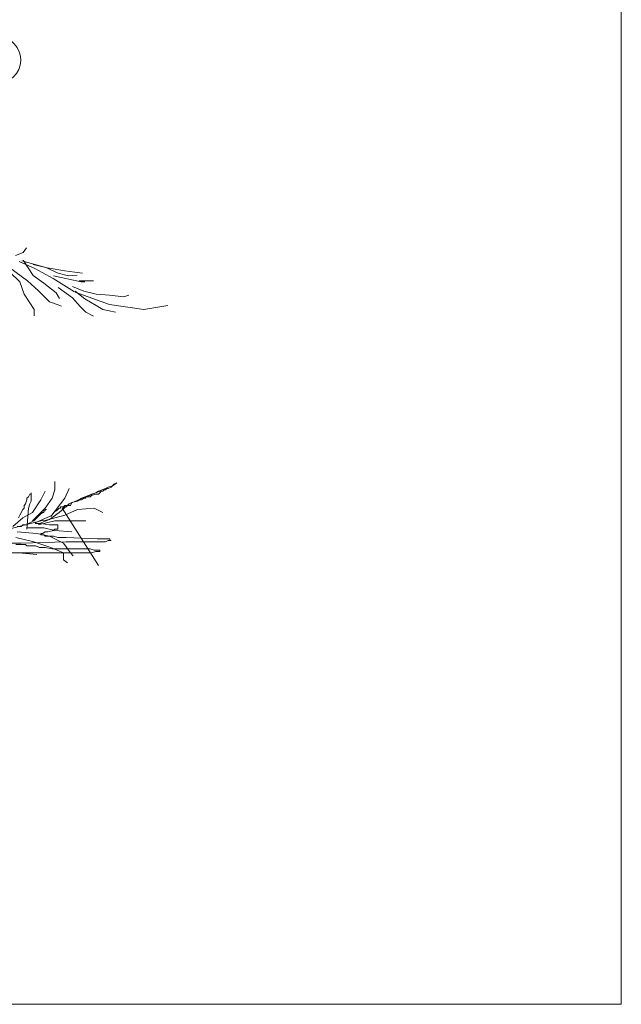
# Model space of a CAD drawing. Units: millimetres. Extents: x 595116 to 630915, y 909473 to 920225.
# Tile 104 of 134: x 629813 to 629825, y 919161 to 919181. Entities that reach past the tile are written whole.
import ezdxf

# ---------------------------------------------------------------- set-up
doc = ezdxf.new("R2010")
doc.units = ezdxf.units.MM
doc.layers.add('L-PLNT', color=85, linetype='Continuous', lineweight=13)

# ---------------------------------------------------------------- blocks, each defined once
blk = doc.blocks.new('A$C4FB75ABC')
for p, q in [((4.6201, 3.4238), (4.6619, 3.4416)), ((4.6619, 3.4416), (4.6798, 3.4655)), ((4.5545, 3.382), (4.6858, 3.2866)), ((4.6395, 3.3917), (4.7247, 3.3534)), ((4.6551, 3.396), (4.7847, 3.3597)), ((4.6619, 3.3999), (4.7156, 3.3164)), ((4.7156, 3.3761), (4.7931, 3.3582)), ((4.5903, 3.3343), (4.644, 3.2807)), ((4.7247, 3.3534), (4.8242, 3.2989)), ((4.7847, 3.3597), (4.8521, 3.3286)), ((4.7931, 3.3582), (4.8886, 3.3403)), ((4.8521, 3.3286), (4.9091, 3.3131)), ((4.8886, 3.3403), (4.9422, 3.3343)), ((4.9422, 3.3343), (4.984, 3.3284)), ((4.644, 3.2807), (4.6679, 3.2151)), ((4.6858, 3.2866), (4.7454, 3.233)), ((4.7156, 3.3164), (4.7752, 3.2747)), ((4.7752, 3.2747), (4.8408, 3.2211)), ((4.8242, 3.2989), (4.9411, 3.2265)), ((4.8262, 3.3131), (4.9765, 3.282)), ((4.9091, 3.3131), (4.9558, 3.3183)), ((4.9661, 3.2866), (5.0079, 3.2866)), ((4.9765, 3.282), (4.9973, 3.282)), ((5.0079, 3.2866), (5.0437, 3.2866)), ((4.6679, 3.2151), (4.6977, 3.1674)), ((4.7454, 3.233), (4.8051, 3.1734)), ((4.8408, 3.2211), (4.8587, 3.1912)), ((4.8521, 3.2509), (4.9299, 3.1939)), ((4.9299, 3.2561), (4.9921, 3.2302)), ((4.9454, 3.2302), (4.9973, 3.1887)), ((4.9454, 3.225), (5.1321, 3.1576)), ((4.9921, 3.2302), (5.0595, 3.2146)), ((5.0595, 3.2146), (5.1321, 3.2094)), ((4.6977, 3.1674), (4.7215, 3.1316)), ((4.8051, 3.1734), (4.8528, 3.1555)), ((4.9299, 3.1939), (4.9713, 3.1472)), ((4.9973, 3.1887), (5.0595, 3.1524)), ((5.1321, 3.2094), (5.2099, 3.1991)), ((5.2099, 3.1991), (5.2358, 3.2094)), ((4.7215, 3.1316), (4.7215, 3.0959)), ((4.8528, 3.1555), (4.8707, 3.1495)), ((4.9713, 3.1472), (5.0025, 3.1162)), ((5.0025, 3.1162), (5.0439, 3.0954)), ((5.0595, 3.1524), (5.0958, 3.1317)), ((5.0958, 3.1317), (5.1632, 3.1162)), ((5.1321, 3.1576), (5.3187, 3.1317)), ((5.3187, 3.1317), (5.4484, 3.1524)), ((4.8198, 2.1038), (4.835, 2.1495)), ((4.835, 2.1495), (4.835, 2.1952)), ((4.8884, 2.1038), (4.9113, 2.1571)), ((5.1095, 2.1571), (5.0714, 2.1419)), ((5.0943, 2.1419), (5.1019, 2.1495)), ((5.1019, 2.1495), (5.1095, 2.1495)), ((5.1248, 2.1648), (5.1095, 2.1571)), ((5.1095, 2.1495), (5.1172, 2.1571)), ((5.1172, 2.1571), (5.1248, 2.1571)), ((5.1477, 2.1724), (5.1248, 2.1648)), ((5.1248, 2.1571), (5.1401, 2.1648)), ((5.1401, 2.1648), (5.1477, 2.1724)), ((5.1477, 2.1724), (5.1629, 2.18)), ((5.1553, 2.18), (5.1477, 2.1724)), ((5.1706, 2.1876), (5.1553, 2.18)), ((5.1629, 2.18), (5.1706, 2.1876)), ((4.6749, 2.0733), (4.6825, 2.0961)), ((4.6825, 2.1038), (4.6901, 2.1114)), ((4.6825, 2.0961), (4.6825, 2.1038)), ((4.6901, 2.1114), (4.6977, 2.1266)), ((4.6977, 2.1266), (4.7054, 2.1266)), ((4.7054, 2.1266), (4.7054, 2.1343)), ((4.7054, 2.1343), (4.7054, 2.0885)), ((4.713, 2.0275), (4.7587, 2.0961)), ((4.7587, 2.0961), (4.7816, 2.1419)), ((4.7816, 2.0504), (4.8198, 2.1038)), ((4.8121, 2.0047), (4.8884, 2.1038)), ((4.9113, 2.0733), (5.079, 2.1419)), ((4.9799, 2.1038), (4.9494, 2.0885)), ((4.957, 2.0885), (4.9723, 2.0961)), ((4.9723, 2.0961), (4.9799, 2.0961)), ((5.018, 2.119), (4.9799, 2.1038)), ((4.9799, 2.0961), (4.9952, 2.1038)), ((4.9952, 2.1038), (5.0028, 2.1038)), ((5.0028, 2.1038), (5.0028, 2.1114)), ((5.0028, 2.1114), (5.0257, 2.1114)), ((5.0333, 2.1266), (5.018, 2.119)), ((5.0257, 2.1114), (5.0333, 2.119)), ((5.0562, 2.1343), (5.0333, 2.1266)), ((5.0333, 2.119), (5.0562, 2.1266)), ((5.0714, 2.1419), (5.0562, 2.1343)), ((5.0562, 2.1266), (5.0714, 2.1266)), ((5.0714, 2.1266), (5.079, 2.1343)), ((5.079, 2.1343), (5.0867, 2.1419)), ((5.0867, 2.1419), (5.0943, 2.1419)), ((4.6444, 2.0123), (4.6596, 2.0428)), ((4.6596, 2.0428), (4.6672, 2.0504)), ((4.6672, 2.0657), (4.6749, 2.0733)), ((4.6672, 2.0504), (4.6672, 2.0657)), ((4.6901, 2.0504), (4.6825, 1.9361)), ((4.6977, 2.0733), (4.6901, 2.0504)), ((4.7054, 2.0885), (4.6977, 2.0733)), ((4.713, 1.9818), (4.7816, 2.0504)), ((4.7816, 2.0352), (4.774, 2.0352)), ((4.774, 2.0352), (4.774, 2.0275)), ((4.7892, 2.0428), (4.7816, 2.0428)), ((4.7816, 2.0428), (4.7816, 2.0352)), ((4.8274, 2.0275), (4.8426, 2.0352)), ((4.8426, 2.0352), (4.8579, 2.0504)), ((4.8579, 2.0275), (4.9113, 2.0733)), ((4.8579, 2.0504), (4.8655, 2.0504)), ((4.8655, 2.0504), (4.8655, 2.058)), ((4.8655, 2.058), (4.8808, 2.058)), ((4.8808, 2.0504), (4.8731, 2.0504)), ((4.8731, 2.0504), (5.0714, 1.7379)), ((4.8808, 2.058), (4.8884, 2.0657)), ((4.896, 2.058), (4.8808, 2.058)), ((4.8808, 2.058), (4.8808, 2.0504)), ((4.8884, 2.0657), (4.9036, 2.0657)), ((4.8884, 2.0123), (4.957, 2.0428)), ((4.9036, 2.0657), (4.896, 2.058)), ((4.9036, 2.0657), (4.9113, 2.0733)), ((4.9189, 2.0657), (4.9036, 2.0657)), ((4.9113, 2.0733), (4.9265, 2.0809)), ((4.9265, 2.0809), (4.9189, 2.0657)), ((4.9265, 2.0809), (4.957, 2.0885)), ((4.9494, 2.0885), (4.9265, 2.0809)), ((4.957, 2.0428), (5.0485, 2.0504)), ((5.0485, 2.0504), (5.0943, 2.0275)), ((4.7725, 1.9851), (4.5975, 1.9398)), ((4.6062, 1.9513), (4.6596, 1.9971)), ((4.6367, 1.9971), (4.6444, 2.0123)), ((4.6596, 1.9971), (4.713, 2.0275)), ((4.7206, 1.9818), (4.7054, 1.9742)), ((4.7359, 1.9971), (4.7206, 1.9818)), ((4.7435, 2.0047), (4.7359, 1.9971)), ((4.7359, 1.9742), (4.7511, 1.9818)), ((4.7511, 2.0123), (4.7435, 2.0047)), ((4.7435, 1.9589), (4.835, 1.9818)), ((4.7664, 2.0275), (4.7511, 2.0123)), ((4.7511, 1.9818), (4.7664, 1.9894)), ((4.7511, 1.9666), (4.8045, 1.9894)), ((4.774, 2.0275), (4.7664, 2.0275)), ((4.7664, 1.9894), (4.8045, 2.0047)), ((4.774, 1.9818), (4.8884, 2.0123)), ((4.8045, 1.9894), (4.8579, 2.0275)), ((4.8045, 2.0047), (4.8198, 2.0123)), ((4.8198, 2.0123), (4.8274, 2.0275)), ((4.835, 1.9818), (4.9494, 1.9818)), ((4.9494, 1.9818), (5.0028, 1.9818)), ((4.652, 1.9513), (4.6291, 1.9513)), ((4.6596, 1.9589), (4.652, 1.9513)), ((4.6825, 1.9589), (4.6596, 1.9589)), ((4.6901, 1.9666), (4.6825, 1.9589)), ((4.6825, 1.9437), (4.774, 1.9437)), ((4.7054, 1.9742), (4.6901, 1.9666)), ((4.7282, 1.9666), (4.7282, 1.9742)), ((4.7282, 1.9742), (4.7359, 1.9742)), ((4.7587, 1.9666), (4.7282, 1.9666)), ((4.8045, 1.9589), (4.7587, 1.9666)), ((4.774, 1.9437), (4.835, 1.9285)), ((4.7969, 1.9208), (4.8274, 1.9285)), ((4.8503, 1.9589), (4.8045, 1.9589)), ((4.8274, 1.9285), (4.835, 1.9361)), ((4.835, 1.9361), (4.8503, 1.9361)), ((4.835, 1.9285), (4.9265, 1.9208)), ((4.8503, 1.9361), (4.8503, 1.9589)), ((4.6215, 1.8903), (4.7206, 1.8675)), ((4.6291, 1.9208), (4.7359, 1.9132)), ((4.7359, 1.9132), (4.8045, 1.898)), ((4.7587, 1.9056), (4.7587, 1.9132)), ((4.7587, 1.9132), (4.7664, 1.9132)), ((4.774, 1.9056), (4.7587, 1.9056)), ((4.7664, 1.9132), (4.7816, 1.9208)), ((4.7816, 1.898), (4.774, 1.9056)), ((4.7816, 1.9208), (4.7969, 1.9208)), ((4.8274, 1.898), (4.7816, 1.898)), ((4.8045, 1.898), (4.8808, 1.8599)), ((4.8503, 1.8903), (4.8274, 1.898)), ((4.896, 1.8903), (4.8503, 1.8903)), ((5.0638, 1.8827), (4.896, 1.8903)), ((5.1324, 1.8827), (5.0638, 1.8827)), ((5.1095, 1.8675), (5.1248, 1.8751)), ((5.1248, 1.8751), (5.1401, 1.8751)), ((5.1324, 1.8751), (5.1324, 1.8827)), ((5.1401, 1.8751), (5.1324, 1.8751)), ((4.591, 1.8599), (4.652, 1.8599)), ((4.6749, 1.8522), (4.6215, 1.8522)), ((4.652, 1.8599), (4.896, 1.8675)), ((4.6825, 1.8446), (4.6749, 1.8522)), ((4.7282, 1.8446), (4.6825, 1.8446)), ((4.7206, 1.8675), (4.8121, 1.837)), ((4.7511, 1.837), (4.7282, 1.8446)), ((4.7816, 1.837), (4.7511, 1.837)), ((4.8198, 1.8294), (4.7816, 1.837)), ((4.8121, 1.837), (4.8808, 1.8065)), ((5.0257, 1.8294), (4.8198, 1.8294)), ((4.8808, 1.8599), (4.9189, 1.8065)), ((4.896, 1.8675), (5.1095, 1.8675)), ((5.0485, 1.8217), (5.0257, 1.8294)), ((5.079, 1.8217), (5.0485, 1.8217)), ((5.079, 1.8141), (5.079, 1.8217)), ((4.1639, 1.8065), (5.0333, 1.8065)), ((4.6367, 1.8065), (4.7359, 1.7989)), ((4.8808, 1.8065), (4.8808, 1.7684)), ((4.8808, 1.7684), (4.9036, 1.7531)), ((4.9189, 1.8065), (4.9341, 1.7913)), ((5.0333, 1.8065), (5.0562, 1.8141)), ((5.0562, 1.8141), (5.079, 1.8141))]:
    blk.add_line(p, q)
blk = doc.blocks.new('A$C77972600')
blk.add_ellipse((5.5155, 1.1693), major_axis=(-0.0941, 0.1005), ratio=0.985729)

msp = doc.modelspace()

# ---------------------------------------------------------------- linework, layer by layer
at = {"layer": 'L-PLNT'}
for p, q in [((629824.951, 919160.917), (629824.951, 919302.009)), ((629511.274, 919160.917), (629824.951, 919160.917))]:
    msp.add_line(p, q, dxfattribs=at)

# ---------------------------------------------------------------- block references
for name, p, xscale, yscale, zscale in [('A$C77972600', (629792.844, 919176.094), 3.512546757812034, 3.512546757812034, 3.512546757812034), ('A$C4FB75ABC', (629795.248, 919163.35), 3.753413438031968, 3.753413438031968, 3.753413438031968)]:
    msp.add_blockref(name, p, dxfattribs=dict(at, xscale=xscale, yscale=yscale, zscale=zscale))

doc.saveas('drawing.dxf')
